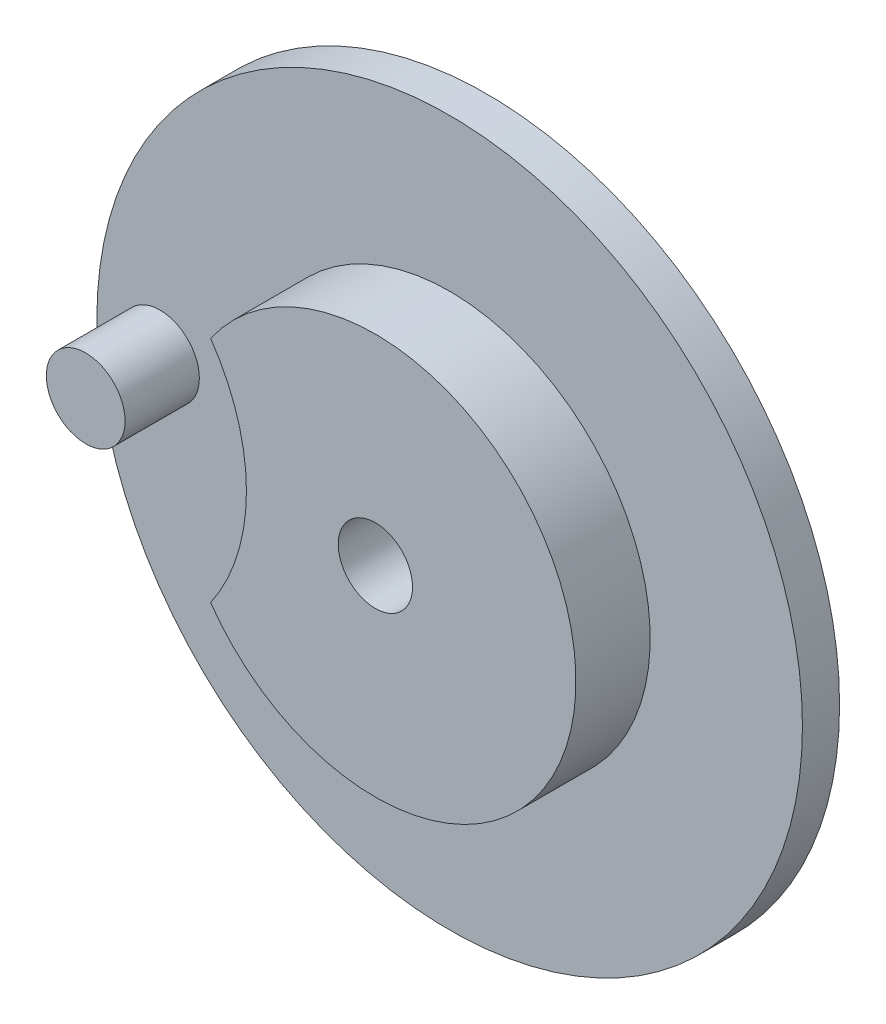
ISO-10303-21;
HEADER;
FILE_DESCRIPTION(('STEP AP214'),'2;1');
FILE_NAME('part.step','',(''),(''),'','','');
FILE_SCHEMA(('AUTOMOTIVE_DESIGN { 1 0 10303 214 1 1 1 1 }'));
ENDSEC;
DATA;
#1=APPLICATION_CONTEXT('core data for automotive mechanical design processes');
#2=APPLICATION_PROTOCOL_DEFINITION('international standard','automotive_design',2000,#1);
#3=PRODUCT_CONTEXT('',#1,'mechanical');
#4=PRODUCT('Part','Part','',(#3));
#5=PRODUCT_RELATED_PRODUCT_CATEGORY('part','',(#4));
#6=PRODUCT_DEFINITION_FORMATION('','',#4);
#7=PRODUCT_DEFINITION_CONTEXT('part definition',#1,'design');
#8=PRODUCT_DEFINITION('design','',#6,#7);
#9=PRODUCT_DEFINITION_SHAPE('','',#8);
#10=(LENGTH_UNIT() NAMED_UNIT(*) SI_UNIT(.MILLI.,.METRE.));
#11=(NAMED_UNIT(*) PLANE_ANGLE_UNIT() SI_UNIT($,.RADIAN.));
#12=(NAMED_UNIT(*) SI_UNIT($,.STERADIAN.) SOLID_ANGLE_UNIT());
#13=UNCERTAINTY_MEASURE_WITH_UNIT(LENGTH_MEASURE(1.E-05),#10,'distance_accuracy_value','');
#14=(GEOMETRIC_REPRESENTATION_CONTEXT(3) GLOBAL_UNCERTAINTY_ASSIGNED_CONTEXT((#13)) GLOBAL_UNIT_ASSIGNED_CONTEXT((#10,
#11,#12)) REPRESENTATION_CONTEXT('',''));
#15=CARTESIAN_POINT('',(0.,0.,0.));
#16=DIRECTION('',(0.,0.,1.));
#17=DIRECTION('',(1.,0.,0.));
#18=AXIS2_PLACEMENT_3D('',#15,#16,#17);
#19=CARTESIAN_POINT('',(0.,0.,5.));
#20=DIRECTION('',(0.,0.,-1.));
#21=DIRECTION('',(-1.,0.,0.));
#22=AXIS2_PLACEMENT_3D('',#19,#20,#21);
#23=CYLINDRICAL_SURFACE('',#22,47.5);
#24=CARTESIAN_POINT('',(0.,0.,5.));
#25=DIRECTION('',(0.,0.,1.));
#26=DIRECTION('',(1.,0.,0.));
#27=AXIS2_PLACEMENT_3D('',#24,#25,#26);
#28=CIRCLE('',#27,47.5);
#29=CARTESIAN_POINT('',(47.5,0.,5.));
#30=VERTEX_POINT('',#29);
#31=EDGE_CURVE('E11',#30,#30,#28,.T.);
#32=ORIENTED_EDGE('',*,*,#31,.F.);
#33=EDGE_LOOP('',(#32));
#34=FACE_BOUND('',#33,.T.);
#35=CARTESIAN_POINT('',(0.,0.,0.));
#36=DIRECTION('',(0.,0.,1.));
#37=DIRECTION('',(1.,0.,0.));
#38=AXIS2_PLACEMENT_3D('',#35,#36,#37);
#39=CIRCLE('',#38,47.5);
#40=CARTESIAN_POINT('',(47.5,0.,0.));
#41=VERTEX_POINT('',#40);
#42=EDGE_CURVE('E45',#41,#41,#39,.T.);
#43=ORIENTED_EDGE('',*,*,#42,.T.);
#44=EDGE_LOOP('',(#43));
#45=FACE_BOUND('',#44,.T.);
#46=ADVANCED_FACE('F39',(#34,#45),#23,.T.);
#47=CARTESIAN_POINT('',(0.,0.,5.));
#48=DIRECTION('',(0.,0.,1.));
#49=DIRECTION('',(1.,0.,0.));
#50=AXIS2_PLACEMENT_3D('',#47,#48,#49);
#51=PLANE('',#50);
#52=CARTESIAN_POINT('',(0.,0.,5.));
#53=DIRECTION('',(0.,0.,1.));
#54=DIRECTION('',(1.,0.,0.));
#55=AXIS2_PLACEMENT_3D('',#52,#53,#54);
#56=CIRCLE('',#55,27.);
#57=CARTESIAN_POINT('',(-22.1792409868759,-15.3974435945089,5.));
#58=VERTEX_POINT('',#57);
#59=CARTESIAN_POINT('',(-22.1792409868759,15.3974435945089,5.));
#60=VERTEX_POINT('',#59);
#61=EDGE_CURVE('E78',#58,#60,#56,.T.);
#62=ORIENTED_EDGE('',*,*,#61,.F.);
#63=CARTESIAN_POINT('',(-44.3584819737518,0.,5.));
#64=DIRECTION('',(0.,0.,1.));
#65=DIRECTION('',(-1.,0.,0.));
#66=AXIS2_PLACEMENT_3D('',#63,#64,#65);
#67=CIRCLE('',#66,27.);
#68=EDGE_CURVE('E56',#58,#60,#67,.T.);
#69=ORIENTED_EDGE('',*,*,#68,.T.);
#70=EDGE_LOOP('',(#62,#69));
#71=FACE_BOUND('',#70,.T.);
#72=CARTESIAN_POINT('',(-39.,0.,5.));
#73=DIRECTION('',(0.,0.,1.));
#74=DIRECTION('',(1.,0.,0.));
#75=AXIS2_PLACEMENT_3D('',#72,#73,#74);
#76=CIRCLE('',#75,5.3);
#77=CARTESIAN_POINT('',(-33.7,0.,5.));
#78=VERTEX_POINT('',#77);
#79=EDGE_CURVE('E77',#78,#78,#76,.T.);
#80=ORIENTED_EDGE('',*,*,#79,.F.);
#81=EDGE_LOOP('',(#80));
#82=FACE_BOUND('',#81,.T.);
#83=ORIENTED_EDGE('',*,*,#31,.T.);
#84=EDGE_LOOP('',(#83));
#85=FACE_BOUND('',#84,.T.);
#86=ADVANCED_FACE('F100',(#71,#82,#85),#51,.T.);
#87=CARTESIAN_POINT('',(0.,0.,0.));
#88=DIRECTION('',(0.,0.,1.));
#89=DIRECTION('',(1.,0.,0.));
#90=AXIS2_PLACEMENT_3D('',#87,#88,#89);
#91=PLANE('',#90);
#92=CARTESIAN_POINT('',(0.,0.,0.));
#93=DIRECTION('',(0.,0.,1.));
#94=DIRECTION('',(1.,0.,0.));
#95=AXIS2_PLACEMENT_3D('',#92,#93,#94);
#96=CIRCLE('',#95,5.);
#97=CARTESIAN_POINT('',(5.,0.,0.));
#98=VERTEX_POINT('',#97);
#99=EDGE_CURVE('E67',#98,#98,#96,.T.);
#100=ORIENTED_EDGE('',*,*,#99,.T.);
#101=EDGE_LOOP('',(#100));
#102=FACE_BOUND('',#101,.T.);
#103=ORIENTED_EDGE('',*,*,#42,.F.);
#104=EDGE_LOOP('',(#103));
#105=FACE_BOUND('',#104,.T.);
#106=ADVANCED_FACE('F94',(#102,#105),#91,.F.);
#107=CARTESIAN_POINT('',(-39.,0.,15.));
#108=DIRECTION('',(0.,0.,-1.));
#109=DIRECTION('',(-1.,0.,0.));
#110=AXIS2_PLACEMENT_3D('',#107,#108,#109);
#111=CYLINDRICAL_SURFACE('',#110,5.3);
#112=CARTESIAN_POINT('',(-39.,0.,15.));
#113=DIRECTION('',(0.,0.,1.));
#114=DIRECTION('',(1.,0.,0.));
#115=AXIS2_PLACEMENT_3D('',#112,#113,#114);
#116=CIRCLE('',#115,5.3);
#117=CARTESIAN_POINT('',(-33.7,0.,15.));
#118=VERTEX_POINT('',#117);
#119=EDGE_CURVE('E85',#118,#118,#116,.T.);
#120=ORIENTED_EDGE('',*,*,#119,.F.);
#121=EDGE_LOOP('',(#120));
#122=FACE_BOUND('',#121,.T.);
#123=ORIENTED_EDGE('',*,*,#79,.T.);
#124=EDGE_LOOP('',(#123));
#125=FACE_BOUND('',#124,.T.);
#126=ADVANCED_FACE('F96',(#122,#125),#111,.T.);
#127=CARTESIAN_POINT('',(-39.,0.,15.));
#128=DIRECTION('',(0.,0.,1.));
#129=DIRECTION('',(1.,0.,0.));
#130=AXIS2_PLACEMENT_3D('',#127,#128,#129);
#131=PLANE('',#130);
#132=ORIENTED_EDGE('',*,*,#119,.T.);
#133=EDGE_LOOP('',(#132));
#134=FACE_BOUND('',#133,.T.);
#135=ADVANCED_FACE('F102',(#134),#131,.T.);
#136=CARTESIAN_POINT('',(0.,0.,15.));
#137=DIRECTION('',(0.,0.,-1.));
#138=DIRECTION('',(-1.,0.,0.));
#139=AXIS2_PLACEMENT_3D('',#136,#137,#138);
#140=CYLINDRICAL_SURFACE('',#139,27.);
#141=ORIENTED_EDGE('',*,*,#61,.T.);
#142=DIRECTION('',(0.,0.,1.));
#143=VECTOR('',#142,1.);
#144=CARTESIAN_POINT('',(-22.1792409868759,15.3974435945089,5.));
#145=LINE('',#144,#143);
#146=CARTESIAN_POINT('',(-22.1792409868759,15.3974435945089,15.));
#147=VERTEX_POINT('',#146);
#148=EDGE_CURVE('E64',#60,#147,#145,.T.);
#149=ORIENTED_EDGE('',*,*,#148,.T.);
#150=CARTESIAN_POINT('',(0.,0.,15.));
#151=DIRECTION('',(0.,0.,1.));
#152=DIRECTION('',(1.,0.,0.));
#153=AXIS2_PLACEMENT_3D('',#150,#151,#152);
#154=CIRCLE('',#153,27.);
#155=CARTESIAN_POINT('',(-22.1792409868759,-15.3974435945089,15.));
#156=VERTEX_POINT('',#155);
#157=EDGE_CURVE('E74',#156,#147,#154,.T.);
#158=ORIENTED_EDGE('',*,*,#157,.F.);
#159=DIRECTION('',(0.,0.,1.));
#160=VECTOR('',#159,1.);
#161=CARTESIAN_POINT('',(-22.1792409868759,-15.3974435945089,5.));
#162=LINE('',#161,#160);
#163=EDGE_CURVE('E52',#58,#156,#162,.T.);
#164=ORIENTED_EDGE('',*,*,#163,.F.);
#165=EDGE_LOOP('',(#141,#149,#158,#164));
#166=FACE_BOUND('',#165,.T.);
#167=ADVANCED_FACE('F71',(#166),#140,.T.);
#168=CARTESIAN_POINT('',(0.,0.,15.));
#169=DIRECTION('',(0.,0.,1.));
#170=DIRECTION('',(1.,0.,0.));
#171=AXIS2_PLACEMENT_3D('',#168,#169,#170);
#172=PLANE('',#171);
#173=CARTESIAN_POINT('',(0.,0.,15.));
#174=DIRECTION('',(0.,0.,1.));
#175=DIRECTION('',(1.,0.,0.));
#176=AXIS2_PLACEMENT_3D('',#173,#174,#175);
#177=CIRCLE('',#176,5.);
#178=CARTESIAN_POINT('',(5.,0.,15.));
#179=VERTEX_POINT('',#178);
#180=EDGE_CURVE('E181',#179,#179,#177,.T.);
#181=ORIENTED_EDGE('',*,*,#180,.F.);
#182=EDGE_LOOP('',(#181));
#183=FACE_BOUND('',#182,.T.);
#184=CARTESIAN_POINT('',(-44.3584819737518,0.,15.));
#185=DIRECTION('',(0.,0.,1.));
#186=DIRECTION('',(-1.,0.,0.));
#187=AXIS2_PLACEMENT_3D('',#184,#185,#186);
#188=CIRCLE('',#187,27.);
#189=EDGE_CURVE('E65',#156,#147,#188,.T.);
#190=ORIENTED_EDGE('',*,*,#189,.F.);
#191=ORIENTED_EDGE('',*,*,#157,.T.);
#192=EDGE_LOOP('',(#190,#191));
#193=FACE_BOUND('',#192,.T.);
#194=ADVANCED_FACE('F76',(#183,#193),#172,.T.);
#195=CARTESIAN_POINT('',(-44.3584819737518,0.,5.));
#196=DIRECTION('',(0.,0.,1.));
#197=DIRECTION('',(1.,0.,0.));
#198=AXIS2_PLACEMENT_3D('',#195,#196,#197);
#199=CYLINDRICAL_SURFACE('',#198,27.);
#200=ORIENTED_EDGE('',*,*,#189,.T.);
#201=ORIENTED_EDGE('',*,*,#148,.F.);
#202=ORIENTED_EDGE('',*,*,#68,.F.);
#203=ORIENTED_EDGE('',*,*,#163,.T.);
#204=EDGE_LOOP('',(#200,#201,#202,#203));
#205=FACE_BOUND('',#204,.T.);
#206=ADVANCED_FACE('F62',(#205),#199,.F.);
#207=CARTESIAN_POINT('',(0.,0.,-15.));
#208=DIRECTION('',(0.,0.,1.));
#209=DIRECTION('',(1.,0.,0.));
#210=AXIS2_PLACEMENT_3D('',#207,#208,#209);
#211=CYLINDRICAL_SURFACE('',#210,5.);
#212=ORIENTED_EDGE('',*,*,#180,.T.);
#213=EDGE_LOOP('',(#212));
#214=FACE_BOUND('',#213,.T.);
#215=ORIENTED_EDGE('',*,*,#99,.F.);
#216=EDGE_LOOP('',(#215));
#217=FACE_BOUND('',#216,.T.);
#218=ADVANCED_FACE('F150',(#214,#217),#211,.F.);
#219=CLOSED_SHELL('',(#46,#86,#106,#126,#135,#167,#194,#206,#218));
#220=MANIFOLD_SOLID_BREP('B2',#219);
#221=ADVANCED_BREP_SHAPE_REPRESENTATION('',(#18,#220),#14);
#222=SHAPE_DEFINITION_REPRESENTATION(#9,#221);
ENDSEC;
END-ISO-10303-21;
